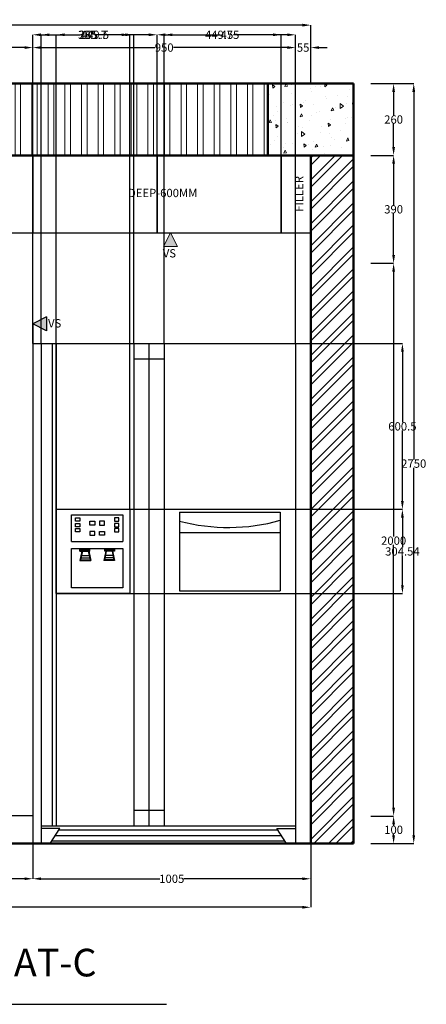
# Model space of a CAD drawing. Units: millimetres. Extents: x 26138 to 44889, y 15820 to 21179.
# Tile 8 of 8: x 43418 to 44889, y 15893 to 19455. Entities that reach past the tile are written whole.
import ezdxf

# ---------------------------------------------------------------- set-up
doc = ezdxf.new("R2010")
doc.units = ezdxf.units.MM
doc.header["$MEASUREMENT"] = 0
doc.header["$PDMODE"] = 3
for name, color, linetype, lineweight in [('A-ANNO-DIMS', 70, 'Continuous', 18), ('A-ANNO-SYMB', 1, 'Continuous', 18), ('A-ANNO-TEXT', 7, 'Continuous', 18), ('A-ELEV', 7, 'Continuous', 25), ('A-FURN-PATT', 40, 'Continuous', 13), ('A-WALL', 1, 'Continuous', 50), ('A-WALL-PATT', 8, 'Continuous', 13)]:
    doc.layers.add(name, color=color, linetype=linetype, lineweight=lineweight)
doc.styles.get("Standard").update_dxf_attribs({"font": 'arial.ttf'})
doc.dimstyles.get("Standard").update_dxf_attribs({"dimtxt": 30, "dimasz": 30, "dimexe": 0.18, "dimexo": 0.0625, "dimgap": 0.09, "dimtad": 0, "dimtih": 1, "dimtoh": 1, "dimdec": 0, "dimzin": 0, "dimdsep": 46, "dimtxsty": 'Standard', "dimcen": 0.09, "dimadec": 0, "dimazin": 0, "dimtfac": 1, "dimtdec": 0, "dimtofl": 0, "dimtmove": 0, "dimatfit": 3, "dimfxl": 1, "dimtolj": 1, "dimtzin": 0, "dimarcsym": 0})

# ---------------------------------------------------------------- blocks, each defined once
blk = doc.blocks.new('*D96')
at = {"layer": 'A-ANNO-DIMS', "color": 0, "lineweight": -2, "transparency": 16777216}
for p, q in [((43015.8, 19224.3), (43015.8, 19354.6)), ((43045.8, 19354.4), (43207, 19354.4)), ((43435.8, 19354.4), (43274.6, 19354.4)), ((43465.8, 19224.3), (43465.8, 19354.6))]:
    blk.add_line(p, q, dxfattribs=at)
at = {"layer": 'A-ANNO-DIMS', "color": 0, "transparency": 16777216}
for points in [[(43045.8, 19359.4), (43045.8, 19349.4), (43015.8, 19354.4)], [(43435.8, 19359.4), (43435.8, 19349.4), (43465.8, 19354.4)]]:
    blk.add_solid(points, dxfattribs=at)
at = {"layer": 'Defpoints', "color": 0, "transparency": 16777216}
for p in [(43465.8, 19354.4), (43015.8, 19224.2), (43465.8, 19224.2)]:
    blk.add_point(p, dxfattribs=at)
at = {"layer": 'A-ANNO-DIMS', "color": 0, "transparency": 16777216, "insert": (43240.8, 19354.4), "char_height": 30, "attachment_point": 5}
blk.add_mtext('\\A1;450', dxfattribs=at)
blk = doc.blocks.new('*D97')
at = {"layer": 'A-ANNO-DIMS', "color": 0, "lineweight": -2, "transparency": 16777216}
for p, q in [((43465.8, 19224.3), (43465.8, 19354.6)), ((43495.8, 19354.4), (43907.6, 19354.4)), ((44385.8, 19354.4), (43974, 19354.4)), ((44415.8, 19224.3), (44415.8, 19354.6))]:
    blk.add_line(p, q, dxfattribs=at)
at = {"layer": 'A-ANNO-DIMS', "color": 0, "transparency": 16777216}
for points in [[(43495.8, 19359.4), (43495.8, 19349.4), (43465.8, 19354.4)], [(44385.8, 19359.4), (44385.8, 19349.4), (44415.8, 19354.4)]]:
    blk.add_solid(points, dxfattribs=at)
at = {"layer": 'Defpoints', "color": 0, "transparency": 16777216}
for p in [(44415.8, 19354.4), (43465.8, 19224.2), (44415.8, 19224.2)]:
    blk.add_point(p, dxfattribs=at)
at = {"layer": 'A-ANNO-DIMS', "color": 0, "transparency": 16777216, "insert": (43940.8, 19354.4), "char_height": 30, "attachment_point": 5}
blk.add_mtext('\\A1;950', dxfattribs=at)
blk = doc.blocks.new('*D98')
at = {"layer": 'A-ANNO-DIMS', "color": 0, "lineweight": -2, "transparency": 16777216}
for p, q in [((44385.8, 19354.4), (44355.8, 19354.4)), ((44415.8, 19224.3), (44415.8, 19354.6)), ((44470.8, 19224.3), (44470.8, 19354.6)), ((44500.8, 19354.4), (44530.8, 19354.4))]:
    blk.add_line(p, q, dxfattribs=at)
at = {"layer": 'A-ANNO-DIMS', "color": 0, "transparency": 16777216}
for points in [[(44385.8, 19359.4), (44385.8, 19349.4), (44415.8, 19354.4)], [(44500.8, 19359.4), (44500.8, 19349.4), (44470.8, 19354.4)]]:
    blk.add_solid(points, dxfattribs=at)
at = {"layer": 'Defpoints', "color": 0, "transparency": 16777216}
for p in [(44470.8, 19354.4), (44415.8, 19224.2), (44470.8, 19224.2)]:
    blk.add_point(p, dxfattribs=at)
at = {"layer": 'A-ANNO-DIMS', "color": 0, "transparency": 16777216, "insert": (44443.3, 19354.4), "char_height": 30, "attachment_point": 5}
blk.add_mtext('\\A1;55', dxfattribs=at)
blk = doc.blocks.new('*D99')
at = {"layer": 'A-ANNO-DIMS', "color": 0, "lineweight": -2, "transparency": 16777216}
for p, q in [((41625.8, 19224.3), (41625.8, 19435.8)), ((41655.8, 19435.6), (42963.6, 19435.6)), ((44440.8, 19435.6), (43054.1, 19435.6)), ((44470.8, 19224.3), (44470.8, 19435.8))]:
    blk.add_line(p, q, dxfattribs=at)
at = {"layer": 'A-ANNO-DIMS', "color": 0, "transparency": 16777216}
for points in [[(41655.8, 19440.6), (41655.8, 19430.6), (41625.8, 19435.6)], [(44440.8, 19440.6), (44440.8, 19430.6), (44470.8, 19435.6)]]:
    blk.add_solid(points, dxfattribs=at)
at = {"layer": 'Defpoints', "color": 0, "transparency": 16777216}
for p in [(41625.8, 19435.6), (41625.8, 19224.2), (44470.8, 19224.2)]:
    blk.add_point(p, dxfattribs=at)
at = {"layer": 'A-ANNO-DIMS', "color": 0, "transparency": 16777216, "insert": (43008.9, 19435.6), "char_height": 30, "attachment_point": 5}
blk.add_mtext('\\A1;2845', dxfattribs=at)
blk = doc.blocks.new('*D100')
at = {"layer": 'A-ANNO-DIMS', "color": 0, "lineweight": -2, "transparency": 16777216}
for p, q in [((44687.8, 19224.2), (44843.4, 19224.2)), ((44843.3, 19194.2), (44843.3, 17864.6)), ((44843.3, 16504.2), (44843.3, 17833.8)), ((44687.8, 16474.2), (44843.4, 16474.2))]:
    blk.add_line(p, q, dxfattribs=at)
at = {"layer": 'A-ANNO-DIMS', "color": 0, "transparency": 16777216}
for points in [[(44838.3, 19194.2), (44848.3, 19194.2), (44843.3, 19224.2)], [(44838.3, 16504.2), (44848.3, 16504.2), (44843.3, 16474.2)]]:
    blk.add_solid(points, dxfattribs=at)
at = {"layer": 'Defpoints', "color": 0, "transparency": 16777216}
for p in [(44687.8, 19224.2), (44687.8, 16474.2), (44843.3, 16474.2)]:
    blk.add_point(p, dxfattribs=at)
at = {"layer": 'A-ANNO-DIMS', "color": 0, "transparency": 16777216, "insert": (44843.3, 17849.2), "char_height": 30, "attachment_point": 5}
blk.add_mtext('\\A1;2750', dxfattribs=at)
blk = doc.blocks.new('*D101')
at = {"layer": 'A-ANNO-DIMS', "color": 0, "lineweight": -2, "transparency": 16777216}
for p, q in [((44687.8, 19224.2), (44770.6, 19224.2)), ((44770.5, 19194.2), (44770.5, 19109.6)), ((44770.5, 18994.2), (44770.5, 19078.8)), ((44687.8, 18964.2), (44770.6, 18964.2))]:
    blk.add_line(p, q, dxfattribs=at)
at = {"layer": 'A-ANNO-DIMS', "color": 0, "transparency": 16777216}
for points in [[(44765.5, 19194.2), (44775.5, 19194.2), (44770.5, 19224.2)], [(44765.5, 18994.2), (44775.5, 18994.2), (44770.5, 18964.2)]]:
    blk.add_solid(points, dxfattribs=at)
at = {"layer": 'Defpoints', "color": 0, "transparency": 16777216}
for p in [(44687.8, 19224.2), (44687.8, 18964.2), (44770.5, 18964.2)]:
    blk.add_point(p, dxfattribs=at)
at = {"layer": 'A-ANNO-DIMS', "color": 0, "transparency": 16777216, "insert": (44770.5, 19094.2), "char_height": 30, "attachment_point": 5}
blk.add_mtext('\\A1;260', dxfattribs=at)
blk = doc.blocks.new('*D102')
at = {"layer": 'A-ANNO-DIMS', "color": 0, "lineweight": -2, "transparency": 16777216}
for p, q in [((44687.8, 18964.2), (44770.6, 18964.2)), ((44770.5, 18934.2), (44770.5, 18784.7)), ((44770.5, 18604.2), (44770.5, 18753.8)), ((44687.8, 18574.2), (44770.6, 18574.2))]:
    blk.add_line(p, q, dxfattribs=at)
at = {"layer": 'A-ANNO-DIMS', "color": 0, "transparency": 16777216}
for points in [[(44765.5, 18934.2), (44775.5, 18934.2), (44770.5, 18964.2)], [(44765.5, 18604.2), (44775.5, 18604.2), (44770.5, 18574.2)]]:
    blk.add_solid(points, dxfattribs=at)
at = {"layer": 'Defpoints', "color": 0, "transparency": 16777216}
for p in [(44687.8, 18964.2), (44687.8, 18574.2), (44770.5, 18574.2)]:
    blk.add_point(p, dxfattribs=at)
at = {"layer": 'A-ANNO-DIMS', "color": 0, "transparency": 16777216, "insert": (44770.5, 18769.2), "char_height": 30, "attachment_point": 5}
blk.add_mtext('\\A1;390', dxfattribs=at)
blk = doc.blocks.new('*D103')
at = {"layer": 'A-ANNO-DIMS', "color": 0, "lineweight": -2, "transparency": 16777216}
for p, q in [((44687.8, 18574.2), (44770.6, 18574.2)), ((44770.5, 18544.2), (44770.5, 17585.9)), ((44770.5, 16604.2), (44770.5, 17555.1)), ((44687.8, 16574.2), (44770.6, 16574.2))]:
    blk.add_line(p, q, dxfattribs=at)
at = {"layer": 'A-ANNO-DIMS', "color": 0, "transparency": 16777216}
for points in [[(44765.5, 18544.2), (44775.5, 18544.2), (44770.5, 18574.2)], [(44765.5, 16604.2), (44775.5, 16604.2), (44770.5, 16574.2)]]:
    blk.add_solid(points, dxfattribs=at)
at = {"layer": 'Defpoints', "color": 0, "transparency": 16777216}
for p in [(44687.8, 18574.2), (44687.8, 16574.2), (44770.5, 16574.2)]:
    blk.add_point(p, dxfattribs=at)
at = {"layer": 'A-ANNO-DIMS', "color": 0, "transparency": 16777216, "insert": (44770.5, 17570.5), "char_height": 30, "attachment_point": 5}
blk.add_mtext('\\A1;2000', dxfattribs=at)
blk = doc.blocks.new('*D104')
at = {"layer": 'A-ANNO-DIMS', "color": 0, "lineweight": -2, "transparency": 16777216}
for p, q in [((44687.8, 16574.2), (44770.6, 16574.2)), ((44770.5, 16544.2), (44770.5, 16539.6)), ((44770.5, 16504.2), (44770.5, 16508.8)), ((44687.8, 16474.2), (44770.6, 16474.2))]:
    blk.add_line(p, q, dxfattribs=at)
at = {"layer": 'A-ANNO-DIMS', "color": 0, "transparency": 16777216}
for points in [[(44765.5, 16544.2), (44775.5, 16544.2), (44770.5, 16574.2)], [(44765.5, 16504.2), (44775.5, 16504.2), (44770.5, 16474.2)]]:
    blk.add_solid(points, dxfattribs=at)
at = {"layer": 'Defpoints', "color": 0, "transparency": 16777216}
for p in [(44687.8, 16574.2), (44687.8, 16474.2), (44770.5, 16474.2)]:
    blk.add_point(p, dxfattribs=at)
at = {"layer": 'A-ANNO-DIMS', "color": 0, "transparency": 16777216, "insert": (44770.5, 16524.2), "char_height": 30, "attachment_point": 5}
blk.add_mtext('\\A1;100', dxfattribs=at)
blk = doc.blocks.new('*D108')
at = {"layer": 'A-ANNO-DIMS', "color": 0, "lineweight": -2, "transparency": 16777216}
for p, q in [((43015.8, 16474.2), (43015.8, 16346.9)), ((43465.8, 16474.2), (43465.8, 16346.9)), ((43045.8, 16347.1), (43207, 16347.1)), ((43435.8, 16347.1), (43274.6, 16347.1))]:
    blk.add_line(p, q, dxfattribs=at)
at = {"layer": 'A-ANNO-DIMS', "color": 0, "transparency": 16777216}
for points in [[(43045.8, 16352.1), (43045.8, 16342.1), (43015.8, 16347.1)], [(43435.8, 16352.1), (43435.8, 16342.1), (43465.8, 16347.1)]]:
    blk.add_solid(points, dxfattribs=at)
at = {"layer": 'Defpoints', "color": 0, "transparency": 16777216}
for p in [(43015.8, 16474.2), (43465.8, 16474.2), (43465.8, 16347.1)]:
    blk.add_point(p, dxfattribs=at)
at = {"layer": 'A-ANNO-DIMS', "color": 0, "transparency": 16777216, "insert": (43240.8, 16347.1), "char_height": 30, "attachment_point": 5}
blk.add_mtext('\\A1;450', dxfattribs=at)
blk = doc.blocks.new('*D109')
at = {"layer": 'A-ANNO-DIMS', "color": 0, "lineweight": -2, "transparency": 16777216}
for p, q in [((43465.8, 16474.2), (43465.8, 16346.9)), ((44470.8, 16474.2), (44470.8, 16346.9)), ((43495.8, 16347.1), (43924.7, 16347.1)), ((44440.8, 16347.1), (44011.9, 16347.1))]:
    blk.add_line(p, q, dxfattribs=at)
at = {"layer": 'A-ANNO-DIMS', "color": 0, "transparency": 16777216}
for points in [[(43495.8, 16352.1), (43495.8, 16342.1), (43465.8, 16347.1)], [(44440.8, 16352.1), (44440.8, 16342.1), (44470.8, 16347.1)]]:
    blk.add_solid(points, dxfattribs=at)
at = {"layer": 'Defpoints', "color": 0, "transparency": 16777216}
for p in [(43465.8, 16474.2), (44470.8, 16474.2), (44470.8, 16347.1)]:
    blk.add_point(p, dxfattribs=at)
at = {"layer": 'A-ANNO-DIMS', "color": 0, "transparency": 16777216, "insert": (43968.3, 16347.1), "char_height": 30, "attachment_point": 5}
blk.add_mtext('\\A1;1005', dxfattribs=at)
blk = doc.blocks.new('*D116')
at = {"layer": 'A-ANNO-DIMS', "color": 0, "lineweight": -2, "transparency": 16777216}
for p, q in [((41625.8, 16474.2), (41625.8, 16243.8)), ((44470.8, 16474.2), (44470.8, 16243.8)), ((41655.8, 16244), (43003, 16244)), ((44440.8, 16244), (43093.5, 16244))]:
    blk.add_line(p, q, dxfattribs=at)
at = {"layer": 'A-ANNO-DIMS', "color": 0, "transparency": 16777216}
for points in [[(41655.8, 16249), (41655.8, 16239), (41625.8, 16244)], [(44440.8, 16249), (44440.8, 16239), (44470.8, 16244)]]:
    blk.add_solid(points, dxfattribs=at)
at = {"layer": 'Defpoints', "color": 0, "transparency": 16777216}
for p in [(41625.8, 16474.2), (44470.8, 16474.2), (44470.8, 16244)]:
    blk.add_point(p, dxfattribs=at)
at = {"layer": 'A-ANNO-DIMS', "color": 0, "transparency": 16777216, "insert": (43048.3, 16244), "char_height": 30, "attachment_point": 5}
blk.add_mtext('\\A1;2845', dxfattribs=at)
blk = doc.blocks.new('SYMB-VS-TRIANGLE')
for p, q in [((0, 0), (25, 49.1)), ((50, 0), (25, 49.1)), ((0, 0), (50, 0))]:
    blk.add_line(p, q)
blk = doc.blocks.new('*D142')
at = {"layer": 'A-ANNO-DIMS', "color": 0, "lineweight": -2, "transparency": 16777216}
for p, q in [((43495.8, 18284.3), (43495.8, 19400.9)), ((43525.8, 19400.7), (43630, 19400.7)), ((43800.8, 19400.7), (43696.6, 19400.7)), ((43830.8, 18284.3), (43830.8, 19400.9))]:
    blk.add_line(p, q, dxfattribs=at)
at = {"layer": 'A-ANNO-DIMS', "color": 0, "transparency": 16777216}
for points in [[(43525.8, 19405.7), (43525.8, 19395.7), (43495.8, 19400.7)], [(43800.8, 19405.7), (43800.8, 19395.7), (43830.8, 19400.7)]]:
    blk.add_solid(points, dxfattribs=at)
at = {"layer": 'Defpoints', "color": 0, "transparency": 16777216}
for p in [(43830.8, 19400.7), (43495.8, 18284.2), (43830.8, 18284.2)]:
    blk.add_point(p, dxfattribs=at)
at = {"layer": 'A-ANNO-DIMS', "color": 0, "transparency": 16777216, "insert": (43663.3, 19400.7), "char_height": 30, "attachment_point": 5}
blk.add_mtext('\\A1;335', dxfattribs=at)
blk = doc.blocks.new('*D143')
at = {"layer": 'A-ANNO-DIMS', "color": 0, "lineweight": -2, "transparency": 16777216}
for p, q in [((43940.8, 18284.3), (43940.8, 19400.9)), ((43970.8, 19400.7), (44144.3, 19400.7)), ((44385.8, 19400.7), (44212.2, 19400.7)), ((44415.8, 18284.3), (44415.8, 19400.9))]:
    blk.add_line(p, q, dxfattribs=at)
at = {"layer": 'A-ANNO-DIMS', "color": 0, "transparency": 16777216}
for points in [[(43970.8, 19405.7), (43970.8, 19395.7), (43940.8, 19400.7)], [(44385.8, 19405.7), (44385.8, 19395.7), (44415.8, 19400.7)]]:
    blk.add_solid(points, dxfattribs=at)
at = {"layer": 'Defpoints', "color": 0, "transparency": 16777216}
for p in [(44415.8, 19400.7), (43940.8, 18284.2), (44415.8, 18284.2)]:
    blk.add_point(p, dxfattribs=at)
at = {"layer": 'A-ANNO-DIMS', "color": 0, "transparency": 16777216, "insert": (44178.3, 19400.7), "char_height": 30, "attachment_point": 5}
blk.add_mtext('\\A1;475', dxfattribs=at)
blk = doc.blocks.new('*D144')
at = {"layer": 'A-ANNO-DIMS', "color": 0, "lineweight": -2, "transparency": 16777216}
for p, q in [((43550.8, 17683.8), (43550.8, 19400.9)), ((43580.8, 19400.7), (43632.7, 19400.7)), ((43786.5, 19400.7), (43734.6, 19400.7)), ((43816.5, 17683.8), (43816.5, 19400.9))]:
    blk.add_line(p, q, dxfattribs=at)
at = {"layer": 'A-ANNO-DIMS', "color": 0, "transparency": 16777216}
for points in [[(43580.8, 19405.7), (43580.8, 19395.7), (43550.8, 19400.7)], [(43786.5, 19405.7), (43786.5, 19395.7), (43816.5, 19400.7)]]:
    blk.add_solid(points, dxfattribs=at)
at = {"layer": 'Defpoints', "color": 0, "transparency": 16777216}
for p in [(43816.5, 19400.7), (43550.8, 17683.8), (43816.5, 17683.8)]:
    blk.add_point(p, dxfattribs=at)
at = {"layer": 'A-ANNO-DIMS', "color": 0, "transparency": 16777216, "insert": (43683.7, 19400.7), "char_height": 30, "attachment_point": 5}
blk.add_mtext('\\A1;265.7', dxfattribs=at)
blk = doc.blocks.new('*D145')
at = {"layer": 'A-ANNO-DIMS', "color": 0, "lineweight": -2, "transparency": 16777216}
for p, q in [((43550.9, 17683.8), (44802.5, 17683.8)), ((44802.3, 17653.8), (44802.3, 17546.9)), ((44802.3, 17409.2), (44802.3, 17516.1)), ((43550.9, 17379.2), (44802.5, 17379.2))]:
    blk.add_line(p, q, dxfattribs=at)
at = {"layer": 'A-ANNO-DIMS', "color": 0, "transparency": 16777216}
for points in [[(44797.3, 17653.8), (44807.3, 17653.8), (44802.3, 17683.8)], [(44797.3, 17409.2), (44807.3, 17409.2), (44802.3, 17379.2)]]:
    blk.add_solid(points, dxfattribs=at)
at = {"layer": 'Defpoints', "color": 0, "transparency": 16777216}
for p in [(43550.8, 17683.8), (43550.8, 17379.2), (44802.3, 17379.2)]:
    blk.add_point(p, dxfattribs=at)
at = {"layer": 'A-ANNO-DIMS', "color": 0, "transparency": 16777216, "insert": (44802.3, 17531.5), "char_height": 30, "attachment_point": 5}
blk.add_mtext('\\A1;304.54', dxfattribs=at)
blk = doc.blocks.new('*D146')
at = {"layer": 'A-ANNO-DIMS', "color": 0, "lineweight": -2, "transparency": 16777216}
for p, q in [((43495.9, 18284.2), (44802.5, 18284.2)), ((44802.3, 18254.2), (44802.3, 17999.4)), ((44802.3, 17713.8), (44802.3, 17968.6)), ((43550.9, 17683.8), (44802.5, 17683.8))]:
    blk.add_line(p, q, dxfattribs=at)
at = {"layer": 'A-ANNO-DIMS', "color": 0, "transparency": 16777216}
for points in [[(44797.3, 18254.2), (44807.3, 18254.2), (44802.3, 18284.2)], [(44797.3, 17713.8), (44807.3, 17713.8), (44802.3, 17683.8)]]:
    blk.add_solid(points, dxfattribs=at)
at = {"layer": 'Defpoints', "color": 0, "transparency": 16777216}
for p in [(43495.8, 18284.2), (43550.8, 17683.8), (44802.3, 17683.8)]:
    blk.add_point(p, dxfattribs=at)
at = {"layer": 'A-ANNO-DIMS', "color": 0, "transparency": 16777216, "insert": (44802.3, 17984), "char_height": 30, "attachment_point": 5}
blk.add_mtext('\\A1;600.5', dxfattribs=at)
blk = doc.blocks.new('*D147')
at = {"layer": 'A-ANNO-DIMS', "color": 0, "lineweight": -2, "transparency": 16777216}
for p, q in [((43465.3, 18684.3), (43465.3, 19400.9)), ((43495.3, 19400.7), (43638.7, 19400.7)), ((43884.9, 19400.7), (43741.5, 19400.7)), ((43914.9, 18684.3), (43914.9, 19400.9))]:
    blk.add_line(p, q, dxfattribs=at)
at = {"layer": 'A-ANNO-DIMS', "color": 0, "transparency": 16777216}
for points in [[(43495.3, 19405.7), (43495.3, 19395.7), (43465.3, 19400.7)], [(43884.9, 19405.7), (43884.9, 19395.7), (43914.9, 19400.7)]]:
    blk.add_solid(points, dxfattribs=at)
at = {"layer": 'Defpoints', "color": 0, "transparency": 16777216}
for p in [(43914.9, 19400.7), (43465.3, 18684.2), (43914.9, 18684.2)]:
    blk.add_point(p, dxfattribs=at)
at = {"layer": 'A-ANNO-DIMS', "color": 0, "transparency": 16777216, "insert": (43690.1, 19400.7), "char_height": 30, "attachment_point": 5}
blk.add_mtext('\\A1;449.5', dxfattribs=at)
blk = doc.blocks.new('*D148')
at = {"layer": 'A-ANNO-DIMS', "color": 0, "lineweight": -2, "transparency": 16777216}
for p, q in [((43914.9, 18684.3), (43914.9, 19400.9)), ((43944.9, 19400.7), (44088.2, 19400.7)), ((44334.4, 19400.7), (44191.1, 19400.7)), ((44364.4, 18684.3), (44364.4, 19400.9))]:
    blk.add_line(p, q, dxfattribs=at)
at = {"layer": 'A-ANNO-DIMS', "color": 0, "transparency": 16777216}
for points in [[(43944.9, 19405.7), (43944.9, 19395.7), (43914.9, 19400.7)], [(44334.4, 19405.7), (44334.4, 19395.7), (44364.4, 19400.7)]]:
    blk.add_solid(points, dxfattribs=at)
at = {"layer": 'Defpoints', "color": 0, "transparency": 16777216}
for p in [(44364.4, 19400.7), (43914.9, 18684.2), (44364.4, 18684.2)]:
    blk.add_point(p, dxfattribs=at)
at = {"layer": 'A-ANNO-DIMS', "color": 0, "transparency": 16777216, "insert": (44139.6, 19400.7), "char_height": 30, "attachment_point": 5}
blk.add_mtext('\\A1;449.5', dxfattribs=at)

msp = doc.modelspace()

# ---------------------------------------------------------------- hatches: boundary and pattern name
at = {"layer": 'A-FURN-PATT'}
h = msp.add_hatch(color=256, dxfattribs=at)
h.dxf.hatch_style = 1
h.paths.add_polyline_path([(43938.774, 18635.141), (43988.774, 18635.141), (43963.774, 18684.233)])
h = msp.add_hatch(color=256, dxfattribs=at)
h.dxf.hatch_style = 1
h.paths.add_polyline_path([(43514.887, 18330.058), (43514.887, 18380.058), (43465.796, 18355.058)])
at = {"layer": 'A-WALL-PATT'}
h = msp.add_hatch(dxfattribs=at)
h.set_pattern_fill('ANSI32', color=256, scale=160, angle=45)
h.set_pattern_definition([(90, (-2438.25, -2020.094), (-60, 0), []), (90, (-2418.25, -2000.094), (-60, 0), [])])
h.paths.add_polyline_path([(44315.796, 18964.233), (44315.796, 19224.233), (41780.796, 19224.233), (41780.796, 19069.233), (41625.796, 19069.233), (41625.796, 18964.233)])
h.paths.add_polyline_path([(42627.517, 19113.099), (43434.744, 19113.099), (43434.744, 19159.664), (42627.517, 19159.664)], flags=24)
h = msp.add_hatch(dxfattribs=at)
h.set_pattern_fill('AR-CONC', color=256, scale=16, angle=45)
h.set_pattern_definition([(95, (-12161.46, -2020.09), (88.24832, 74.04913), [12, -132]), (40, (-12161.46, -2020.09), (-100.79875, 69.4029), [9.6, -105.6]), (145.45144, (-12154.11, -2013.92), (-12.55043, 143.45204), [10.19843, -112.18274]), (91.1842, (-12184.09, -1997.47), (139.47094, 102.0182), [18, -198]), (141.63564, (-12172.47, -1988.96), (-4.464, 215.95387), [15.29765, -168.2742]), (36.18416, (-12184.09, -1997.47), (-4.464, 215.95387), [14.4, -158.4]), (66, (-12167.12, -1991.81), (113.08345, 21.9812), [12, -132]), (11, (-12167.12, -1991.81), (-54.51337, 109.56935), [9.6, -105.6]), (116.45144, (-12157.7, -1989.98), (58.57008, 131.55054), [10.19843, -112.18274]), (82.5, (-12161.462, -2020.094), (-36.28691, 39.03837), [0, -104.32, 0, -107.2, 0, -106]), (52.5, (-12161.46, -2020.094), (-14.85967, 74.38551), [0, -61.12, 0, -101.92, 0, -40.4]), (12.5, (-12186.69, -2045.323), (62.946907, 57.843322), [0, -40, 0, -124.8, 0, -165.6]), (2.5, (-12198.005, -2056.64), (54.6544, 77.30557), [0, -52, 0, -82.88, 0, -117.6])])
h.paths.add_polyline_path([(44470.796, 19224.233), (44315.796, 19224.233), (44315.796, 18964.233), (44470.796, 18964.233), (44625.796, 18964.469), (44625.796, 19224.233)])
h = msp.add_hatch(dxfattribs=at)
h.set_pattern_fill('ANSI32', color=256, scale=150)
h.set_pattern_definition([(45, (-2438.253, -2020.094), (-39.774756, 39.774756), []), (45, (-2411.736, -2020.094), (-39.774756, 39.774756), [])])
h.paths.add_polyline_path([(44625.796, 18964.469), (44470.796, 18964.233), (44470.796, 16474.233), (44625.796, 16474.233)])

# ---------------------------------------------------------------- linework, layer by layer
at = {"layer": 'A-ELEV'}
for p, q in [((43465.334, 18964.233), (43465.334, 18684.233)), ((43465.796, 18284.233), (43465.334, 18964.233)), ((43914.873, 18964.233), (43914.873, 18684.233)), ((43914.873, 18684.233), (43914.873, 18964.233)), ((44364.412, 18964.233), (44364.412, 18684.233)), ((43015.796, 18684.233), (44470.796, 18684.233)), ((43514.887, 18380.058), (43465.796, 18355.058)), ((43514.887, 18330.058), (43465.796, 18355.058)), ((43465.796, 18355.058), (43465.796, 16474.233)), ((43514.887, 18380.058), (43514.887, 18330.058)), ((43465.796, 18284.233), (44415.796, 18284.233)), ((43495.796, 18284.233), (43495.796, 16474.233)), ((43535.796, 18284.233), (43535.796, 16539.233)), ((43550.796, 18284.233), (43550.796, 16539.233)), ((43830.796, 18284.233), (43830.796, 16539.233)), ((43885.796, 18284.233), (43885.796, 16539.233)), ((43940.796, 18284.233), (43940.796, 16539.233)), ((44415.796, 18284.233), (44415.796, 16474.233)), ((43830.796, 18228.195), (43940.796, 18228.195)), ((43550.796, 17683.769), (43816.517, 17683.769)), ((43550.796, 17379.233), (43550.796, 17683.769)), ((43816.517, 17683.769), (43816.517, 17379.233)), ((43940.796, 17683.769), (44415.796, 17683.769)), ((43940.796, 17683.769), (43940.796, 17379.233)), ((43995.796, 17673.769), (43995.796, 17389.233)), ((43995.796, 17673.769), (44360.796, 17673.769)), ((44360.796, 17673.769), (44360.796, 17389.233)), ((44415.796, 17683.769), (44415.796, 17379.233)), ((43605.796, 17663.769), (43791.517, 17663.769)), ((43605.796, 17567.174), (43605.796, 17663.769)), ((43791.517, 17663.769), (43791.517, 17567.174)), ((43995.796, 17599.943), (44360.796, 17599.943)), ((43605.796, 17567.174), (43791.517, 17567.174)), ((43605.796, 17399.233), (43605.796, 17542.174)), ((43605.796, 17542.174), (43791.517, 17542.174)), ((43635.884, 17532.174), (43635.884, 17542.174)), ((43635.884, 17537.174), (43671.545, 17537.174)), ((43635.884, 17532.174), (43671.545, 17532.174)), ((43643.109, 17532.174), (43635.898, 17499.082)), ((43645.156, 17532.174), (43638.381, 17501.082)), ((43665.885, 17532.174), (43672.661, 17501.082)), ((43667.932, 17532.174), (43675.144, 17499.082)), ((43671.545, 17532.174), (43671.545, 17542.174)), ((43729.381, 17532.174), (43722.169, 17499.082)), ((43731.428, 17532.174), (43724.652, 17501.082)), ((43725.768, 17532.174), (43725.768, 17542.174)), ((43761.429, 17537.174), (43725.768, 17537.174)), ((43761.429, 17532.174), (43725.768, 17532.174)), ((43752.157, 17532.174), (43758.932, 17501.082)), ((43754.204, 17532.174), (43761.415, 17499.082)), ((43761.429, 17542.174), (43761.429, 17532.174)), ((43791.517, 17542.174), (43791.517, 17399.233)), ((43635.898, 17499.082), (43675.144, 17499.082)), ((43638.381, 17501.082), (43672.661, 17501.082)), ((43639.997, 17508.5), (43671.044, 17508.502)), ((43641.768, 17516.628), (43669.273, 17516.628)), ((43761.415, 17499.082), (43722.169, 17499.082)), ((43758.932, 17501.082), (43724.652, 17501.082)), ((43757.316, 17508.5), (43726.269, 17508.502)), ((43755.545, 17516.628), (43728.04, 17516.628)), ((43791.517, 17399.233), (43605.796, 17399.233)), ((43995.796, 17389.233), (44360.796, 17389.233)), ((43816.517, 17379.233), (43550.796, 17379.233)), ((43940.796, 17379.233), (44415.796, 17379.233)), ((43465.796, 16574.233), (41625.796, 16574.233)), ((43830.796, 16595.271), (43940.796, 16595.271)), ((43495.796, 16539.233), (44415.796, 16539.233)), ((43562.989, 16529.146), (43495.796, 16529.146)), ((43528.255, 16474.233), (43562.989, 16529.146)), ((43547.231, 16504.233), (44364.36, 16504.233)), ((43559.881, 16524.233), (44351.71, 16524.233)), ((44383.336, 16474.233), (44348.603, 16529.146)), ((44348.603, 16529.146), (44415.796, 16529.146)), ((43534.58, 16484.233), (44377.011, 16484.233)), ((41936.11, 15892.9), (43949.787, 15892.9))]:
    msp.add_line(p, q, dxfattribs=at)
for points in [[(43620.5, 17652.997), (43636.256, 17652.997), (43636.256, 17641.188), (43620.5, 17641.188)], [(43672.003, 17641.201), (43690.095, 17641.201), (43690.095, 17627.033), (43672.003, 17627.033)], [(43725.309, 17641.201), (43707.218, 17641.201), (43707.218, 17627.033), (43725.309, 17627.033)], [(43776.813, 17652.997), (43761.057, 17652.997), (43761.057, 17641.188), (43776.813, 17641.188)], [(43620.5, 17632.753), (43636.256, 17632.753), (43636.256, 17620.944), (43620.5, 17620.944)], [(43620.5, 17614.196), (43636.256, 17614.196), (43636.256, 17602.386), (43620.5, 17602.386)], [(43672.003, 17589.742), (43690.095, 17589.742), (43690.095, 17603.911), (43672.003, 17603.911)], [(43725.309, 17589.742), (43707.218, 17589.742), (43707.218, 17603.911), (43725.309, 17603.911)], [(43776.813, 17632.753), (43761.057, 17632.753), (43761.057, 17620.944), (43776.813, 17620.944)], [(43776.813, 17614.196), (43761.057, 17614.196), (43761.057, 17602.386), (43776.813, 17602.386)]]:
    msp.add_lwpolyline(points, close=True, dxfattribs=at)
msp.add_arc((44173.431, 18308.707), 690.45, 255.091535, 285.745525, dxfattribs=at)
at = {"layer": 'A-WALL'}
for p, q in [((41470.796, 19224.233), (44470.796, 19224.233)), ((44315.796, 18964.233), (44315.796, 19224.233)), ((44470.796, 19224.233), (44625.796, 19224.233)), ((44625.796, 19224.233), (44625.796, 19069.233)), ((44625.796, 19069.233), (44625.796, 16474.233)), ((44470.796, 18964.233), (41625.796, 18964.233)), ((44470.796, 18964.233), (44315.796, 18964.233)), ((44625.796, 18964.469), (44470.796, 18964.233)), ((44470.796, 18964.233), (44470.796, 16474.233)), ((44470.796, 16474.233), (41470.796, 16474.233)), ((44625.796, 16474.233), (44470.796, 16474.233))]:
    msp.add_line(p, q, dxfattribs=at)

# ---------------------------------------------------------------- block references
at = {"layer": 'A-ANNO-SYMB'}
msp.add_blockref('SYMB-VS-TRIANGLE', (43938.774, 18635.141), dxfattribs=at)

# ---------------------------------------------------------------- texts
at = {"layer": 'A-ANNO-TEXT'}
msp.add_text('FILLER', height=30, rotation=90, dxfattribs=at).set_placement((44443.446, 18760.331))
for s, height, p in [('DEEP-600MM ', 30, (43809.753, 18813.375)), ('VS', 30, (43935.738, 18595.087)), ('VS', 30, (43520.919, 18341.842)), ('KITCHEN ELEVATION AT-C', 100, (42043.106, 15993.854))]:
    msp.add_text(s, height=height, dxfattribs=at).set_placement(p)

# ---------------------------------------------------------------- dimensions: what is measured, and where the dimension line sits
at = {"layer": 'A-ANNO-DIMS'}
for base, p1, p2, picture, middle in [((41625.796, 19435.636), (44470.796, 19224.233), (41625.796, 19224.233), '*D99', (43008.876, 19435.636)), ((44470.796, 16244.003), (41625.796, 16474.233), (44470.796, 16474.233), '*D116', (43048.296, 16244.003))]:
    dim = msp.add_linear_dim(base=base, p1=p1, p2=p2, dimstyle='Standard', override={"dimclrd": 0, "dimclre": 0, "dimclrt": 0}, dxfattribs=at)
    dim.commit()
    dim.dimension.update_dxf_attribs({"geometry": picture, "text_midpoint": middle, "dimtype": 160})
for base, p1, p2, override, picture, middle in [((43914.873, 19400.733), (43465.334, 18684.233), (43914.873, 18684.233), {"dimdec": 1, "dimlfac": 1, "dimrnd": 0, "dimzin": 0, "dimdsep": 46, "dimlunit": 2}, '*D147', (43690.104, 19400.733)), ((43830.796, 19400.733), (43495.796, 18284.233), (43830.796, 18284.233), {"dimdec": 0, "dimlfac": 1, "dimrnd": 0, "dimzin": 0, "dimdsep": 46, "dimlunit": 2}, '*D142', (43663.296, 19400.733)), ((43816.517, 19400.733), (43550.796, 17683.769), (43816.517, 17683.769), {"dimdec": 1, "dimlfac": 1, "dimrnd": 0, "dimzin": 0, "dimdsep": 46, "dimlunit": 2}, '*D144', (43683.656, 19400.733)), ((44364.412, 19400.733), (43914.873, 18684.233), (44364.412, 18684.233), {"dimdec": 1, "dimlfac": 1, "dimrnd": 0, "dimzin": 0, "dimdsep": 46, "dimlunit": 2}, '*D148', (44139.642, 19400.733)), ((44415.796, 19400.733), (43940.796, 18284.233), (44415.796, 18284.233), {"dimdec": 0, "dimlfac": 1, "dimrnd": 0, "dimzin": 0, "dimdsep": 46, "dimlunit": 2}, '*D143', (44178.296, 19400.733)), ((43465.796, 19354.4), (43015.796, 19224.233), (43465.796, 19224.233), {"dimclrd": 0, "dimclre": 0, "dimclrt": 0}, '*D96', (43240.796, 19354.4)), ((44415.796, 19354.4), (43465.796, 19224.233), (44415.796, 19224.233), {"dimclrd": 0, "dimclre": 0, "dimclrt": 0}, '*D97', (43940.796, 19354.4)), ((44470.796, 19354.4), (44415.796, 19224.233), (44470.796, 19224.233), {"dimclrd": 0, "dimclre": 0, "dimclrt": 0}, '*D98', (44443.296, 19354.4)), ((43465.796, 16347.119), (43015.796, 16474.233), (43465.796, 16474.233), {"dimclrd": 0, "dimclre": 0, "dimclrt": 0}, '*D108', (43240.796, 16347.119)), ((44470.796, 16347.119), (43465.796, 16474.233), (44470.796, 16474.233), {"dimclrd": 0, "dimclre": 0, "dimclrt": 0}, '*D109', (43968.296, 16347.119))]:
    dim = msp.add_linear_dim(base=base, p1=p1, p2=p2, dimstyle='Standard', override=override, dxfattribs=at)
    dim.commit()
    dim.dimension.update_dxf_attribs({"geometry": picture, "text_midpoint": middle})
for base, p1, p2, picture, middle in [((44843.254, 16474.233), (44687.758, 19224.233), (44687.758, 16474.233), '*D100', (44843.254, 17849.233)), ((44770.454, 16574.233), (44687.758, 18574.233), (44687.758, 16574.233), '*D103', (44770.454, 17570.508))]:
    dim = msp.add_linear_dim(base=base, p1=p1, p2=p2, angle=90, dimstyle='Standard', override={"dimclrd": 0, "dimclre": 0, "dimclrt": 0}, dxfattribs=at)
    dim.commit()
    dim.dimension.update_dxf_attribs({"geometry": picture, "text_midpoint": middle, "dimtype": 160})
for base, p1, p2, override, picture, middle in [((44770.454, 18964.233), (44687.758, 19224.233), (44687.758, 18964.233), {"dimclrd": 0, "dimclre": 0, "dimclrt": 0}, '*D101', (44770.454, 19094.233)), ((44770.454, 18574.233), (44687.758, 18964.233), (44687.758, 18574.233), {"dimclrd": 0, "dimclre": 0, "dimclrt": 0}, '*D102', (44770.454, 18769.233)), ((44802.296, 17683.769), (43495.796, 18284.233), (43550.796, 17683.769), {"dimdec": 1, "dimlfac": 1, "dimrnd": 0, "dimzin": 0, "dimdsep": 46, "dimlunit": 2}, '*D146', (44802.296, 17984.001)), ((44802.296, 17379.233), (43550.796, 17683.769), (43550.796, 17379.233), {"dimdec": 2, "dimlfac": 1, "dimrnd": 0, "dimzin": 0, "dimdsep": 46, "dimlunit": 2}, '*D145', (44802.296, 17531.501)), ((44770.454, 16474.233), (44687.758, 16574.233), (44687.758, 16474.233), {"dimclrd": 0, "dimclre": 0, "dimclrt": 0}, '*D104', (44770.454, 16524.233))]:
    dim = msp.add_linear_dim(base=base, p1=p1, p2=p2, angle=90, dimstyle='Standard', override=override, dxfattribs=at)
    dim.commit()
    dim.dimension.update_dxf_attribs({"geometry": picture, "text_midpoint": middle})

doc.saveas('drawing.dxf')
